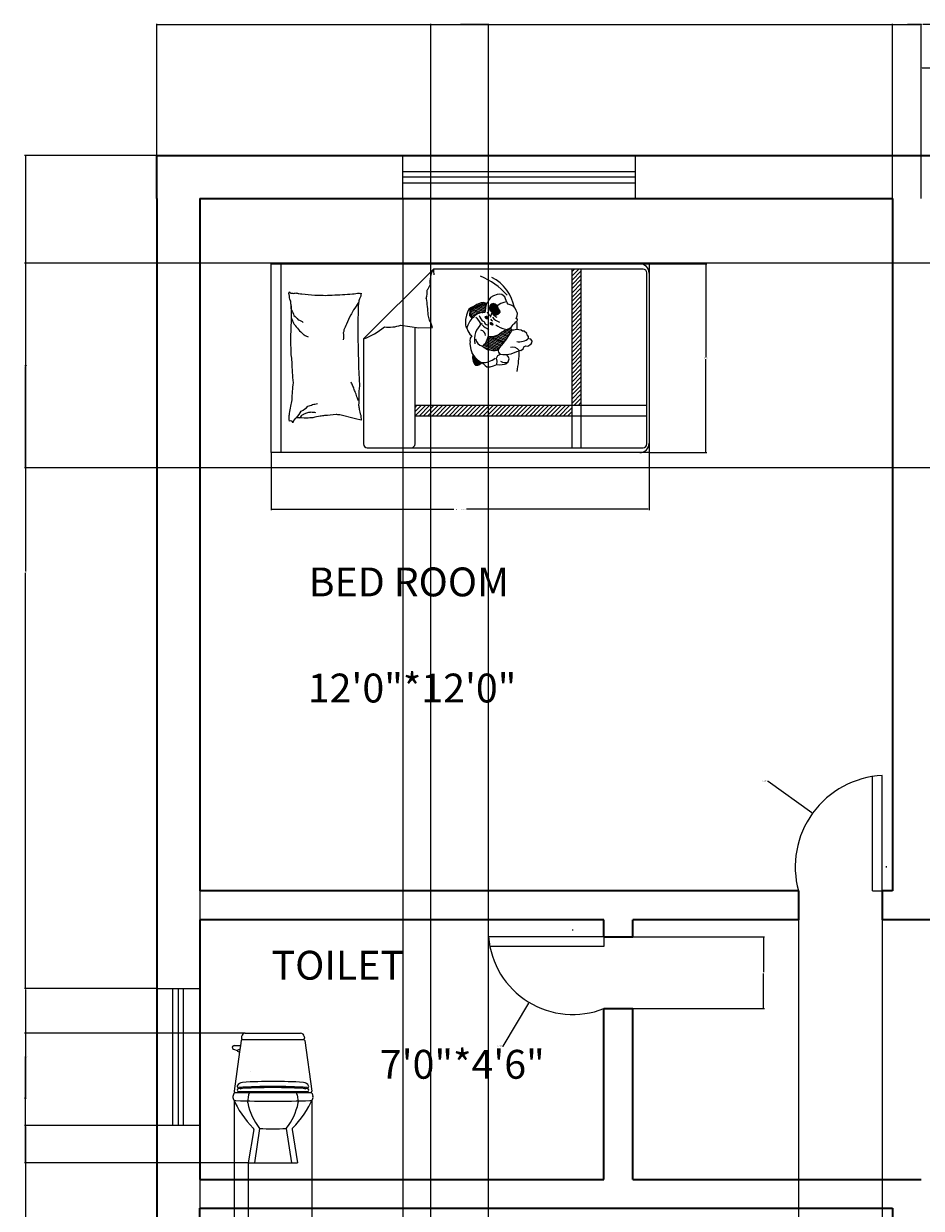
# Model space of a CAD drawing. Units: inches. Extents: x -17 to 1735, y -531 to 60.
# Tile 3 of 27: x -17 to 170, y -187 to 60. Entities that reach past the tile are written whole.
import ezdxf

# ---------------------------------------------------------------- set-up
doc = ezdxf.new("R2010")
doc.units = ezdxf.units.IN
doc.header["$MEASUREMENT"] = 0
for name, color, linetype, lineweight in [('A-ANNO-DIMS', 2, 'Continuous', 18), ('A-AREA-IDEN', 7, 'Continuous', 25), ('A-DOOR', 4, 'Continuous', 18), ('A-GLAZ', 4, 'Continuous', 18), ('A-WALL', 7, 'Continuous', 35)]:
    doc.layers.add(name, color=color, linetype=linetype, lineweight=lineweight)
for name, color, linetype, lineweight, true_color in [('A-FURN', 242, 'Continuous', 18, 0xcd2027), ('WC-Detail_dwgmodels.com', 30, 'Continuous', 13, 0xf8991e), ('WC-Outline_dwgmodels.com', 30, 'Continuous', 18, 0xf8991e)]:
    doc.layers.add(name, color=color, linetype=linetype, lineweight=lineweight, true_color=true_color)
doc.styles.get("Standard").update_dxf_attribs({"font": 'arial.ttf'})
doc.dimstyles.get("Standard").update_dxf_attribs({"dimtxt": 0.18, "dimasz": 0.18, "dimexe": 0.18, "dimexo": 0.0625, "dimgap": 0.09, "dimtad": 0, "dimtih": 1, "dimtoh": 1, "dimdec": 4, "dimzin": 0, "dimdsep": 46, "dimtxsty": 'Standard', "dimcen": 0.09, "dimadec": 0, "dimazin": 0, "dimtfac": 1, "dimtdec": 4, "dimtofl": 0, "dimtmove": 0, "dimatfit": 3, "dimfxl": 1, "dimtolj": 1, "dimtzin": 0, "dimarcsym": 0})

# ---------------------------------------------------------------- blocks, each defined once
blk = doc.blocks.new('BED-SINGLE-PLAN')
h = blk.add_hatch()
h.set_pattern_fill('ANSI31', color=256, scale=0.196463, angle=90, style=0)
h.set_pattern_definition([(225, (-27.0618, 48.5235), (-0.4410725, 0.4410725), [])])
h.paths.add_polyline_path([(62.55, 9.8), (29.91, 9.8), (29.91, 7.6), (62.55, 7.6)])
h.paths.add_polyline_path([(62.55, 9.8), (64.48, 9.8), (64.48, 38.18), (62.55, 38.18)])
h = blk.add_hatch()
h.set_pattern_fill('ANSI31', color=256, scale=2.357559, angle=112.8083, style=0)
h.set_pattern_definition([(157.808265, (-756.06988, 363.93155), (-0.11130837, -0.27286535), [])])
h.paths.add_polyline_path([(42.9, 28.85), (43.53, 29.05), (44.41, 29.13), (44.47, 29.42), (44.54, 30.16), (44.69, 30.7), (44.07, 30.85), (43.35, 30.52), (41.94, 30.01), (41.58, 29.54), (41.52, 28.62), (41.97, 28.11), (42.32, 28.49)])
h.paths.add_polyline_path([(45.09, 24.15, -0.19505), (43.9, 22.11, 0.242355), (47, 21.35, 0.070869), (50.1, 25.47), (49.89, 25.73), (49.62, 25.88), (48.82, 25.54), (47.87, 25.05), (47.21, 24.51), (46.36, 24.21)])
h = blk.add_hatch()
h.set_pattern_fill('ANSI31', color=256, scale=1.392433, angle=112.8083, style=0)
h.set_pattern_definition([(157.808265, (-714.60694, 367.20017), (-0.065741506, -0.161161097), [])])
h.paths.add_polyline_path([(45.75, 29.39), (46.01, 28.9), (46.14, 28.75), (46.34, 28.64), (46.5, 28.59), (46.86, 28.63), (47.26, 28.84), (47.59, 29.2), (47.52, 29.53), (47.21, 29.96), (47.12, 30.29), (46.97, 30.53), (46.54, 30.87), (46.19, 31), (45.76, 30.88), (45.45, 30.56), (45.37, 30.21), (45.4, 29.92), (45.54, 29.52)])
h = blk.add_hatch()
h.set_pattern_fill('ANSI31', color=256, scale=0.556973, angle=112.8083, style=0)
h.set_pattern_definition([(157.808265, (-714.60694, 367.20017), (-0.0262966024, -0.0644644387), [])])
h.paths.add_polyline_path([(45.8, 27.02), (45.59, 27), (45.47, 26.92), (45.58, 26.73), (45.73, 26.62), (46.03, 26.56), (46.14, 26.64), (46.08, 26.8), (45.97, 26.95)])
h.paths.add_polyline_path([(44.84, 28.32), (44.68, 28.33), (44.51, 28.27), (44.45, 28.18), (44.46, 28.11), (44.56, 28.01), (44.67, 27.9), (44.88, 27.87), (45.01, 27.95), (45.02, 28.12)])
h = blk.add_hatch()
h.set_pattern_fill('ANSI31', color=256, scale=1.178779, angle=112.8083, style=0)
h.set_pattern_definition([(157.808265, (-756.06988, 363.93155), (-0.055654185, -0.136432674), [])])
h.paths.add_polyline_path([(41.9, 20.41), (41.91, 20.39), (41.88, 19.75), (42, 19.04), (42.19, 18.52), (42.51, 18.19), (42.99, 18.18), (43.33, 18.35), (43.64, 18.6), (43.79, 18.72, -0.129501)])
for p, q in [((0, 39.29), (78.59, 39.29)), ((0, 0), (0, 39.29)), ((2.06, 0), (2.06, 39.29)), ((19.2, 23.68), (33.73, 38.18)), ((77.32, 38.18), (33.73, 38.18)), ((62.55, 1.01), (62.55, 38.18)), ((64.48, 1.01), (64.48, 38.18)), ((78.11, 1.8), (78.11, 37.39)), ((78.59, 39.29), (78.59, 0)), ((29.91, 1.8), (29.91, 26.11)), ((19.2, 23.68), (19.2, 1.8)), ((78.59, 0), (0, 0)), ((19.98, 1.01), (77.32, 1.01))]:
    blk.add_line(p, q)
for points in [[(5.25, 7.27, 0.263368), (4.51, 6.17, 0.494818), (3.78, 6.53, 0.049225), (3.71, 7.23, 0.036831), (3.78, 8.16, 0.031893), (4.1, 9.65, -0.035782), (4.37, 10.98, -0.032941), (4.6, 14.51, -0.026564), (4.37, 18.88, -0.017905), (4.16, 20.35, 0.009667), (4.07, 23.11, 0.03204), (4.1, 24.57, -0.018442), (4.22, 27.09, -0.010837), (4.19, 29.64, -0.014624), (4.07, 31.52, -0.111249), (3.78, 32.41, 0.153708), (3.63, 33.07, 0.076444), (3.7, 33.36, 0.215512), (3.78, 33.44, 0.585858), (3.9, 33.33, -0.363489), (4, 33.14, -0.191716), (4.45, 33.14, 0.129675), (5.1, 33.22, 0.01735), (5.76, 33.1, -0.019326), (6.36, 33, -0.018818), (9.04, 32.74, -0.021828), (11.37, 32.7, -0.006204), (12.7, 32.76, -0.001963), (16.9, 33, -0.028341), (18.32, 33.16, 0.117014), (18.67, 33.14, 0.36606), (18.71, 33.09, 0.03973), (18.6, 32.55, 0.048309), (18.38, 32.01, -0.062981), (18.23, 31.59, -0.04058), (18.09, 30.67, -0.014345), (18.01, 28.05, -0.005484), (18.04, 23.12, -0.004707), (18.15, 17.38, -0.008762), (18.26, 15.71, 0.008153), (18.38, 13.91, 0.06251), (18.2, 11.67, -0.078669), (18.12, 9.88, -0.047825), (18.31, 9, 0.034494), (18.6, 7.79, 0.023571), (18.71, 6.79, 0.510228), (18.67, 6.76), (17.49, 7.05), (14.25, 7.86, -0.073041), (13.48, 7.94, -0.023305), (11.08, 7.72, -0.018299), (10.18, 7.56, 0.01097), (8.68, 7.27, 0.042281), (7.34, 7.15, 0.027201), (5.24, 7.27)], [(4, 31.08, -0.088153), (4.14, 29.72, -0.088153), (4.73, 28.5, -0.077547), (5.58, 27.64, -0.077547), (6.65, 27.09)], [(18.15, 31.23, -0.016108), (17.12, 29.7, -0.024599), (16.53, 28.64, -0.009477), (15.62, 26.72, -0.015937), (15.13, 25.54, -0.072521), (14.99, 24.9, -0.033339), (14.98, 23.48)], [(4.22, 27.86, -0.027842), (4.64, 26.92, -0.048685), (4.96, 26.43, -0.023666), (5.91, 25.33, -0.031223), (6.72, 24.58, -0.046801), (7.03, 24.38, -0.023191), (7.68, 24.07)], [(19.2, 23.68, 0.085272), (23.52, 26.17, 0.124044), (26.96, 26.53), (30.71, 25.99), (33.56, 26.06)], [(18.09, 10.82, -0.009729), (17.74, 11.9, -0.009729), (17.34, 12.95, -0.007971), (16.99, 13.81, -0.007971), (16.61, 14.65)], [(5.25, 7.27, 0.077379), (6.25, 8.63, 0.077379), (7.61, 9.63, 0.047525), (8.58, 10.02, 0.047525), (9.6, 10.22)], [(5.88, 7.21, 0.05369), (6.39, 7.77, 0.070312), (6.87, 8.08, 0.015448), (7.21, 8.23, 0.013244), (7.61, 8.38, 0.082127), (8.32, 8.5, 0.064164), (9.23, 8.38)]]:
    blk.add_lwpolyline(points, format="xyb")
for points in [[(43.79, 18.72), (44.04, 18.56), (44.46, 18.12), (44.86, 17.87), (45.53, 17.83), (46.24, 18.04), (46.92, 18.32), (47.57, 18.24), (48.51, 18.4), (48.81, 18.47), (49.3, 18.91), (49.47, 19.49), (49.29, 19.97), (48.92, 20.38), (49.91, 20.56), (51.05, 21.01), (51.55, 21.16), (51.59, 21.33), (51.88, 21.27), (52.46, 21.66), (52.55, 22), (52.94, 22.19), (53.35, 22.15), (53.8, 22.4), (54.07, 22.6), (54.21, 22.84), (54.27, 23.19), (53.95, 23.59), (53.59, 23.67), (53.53, 23.82), (53.51, 24.14), (53.22, 24.49), (53.14, 24.75), (52.57, 25.26), (52.25, 25.24), (51.94, 25.49), (50.98, 25.59), (50.47, 25.47), (50.13, 25.44), (49.89, 25.73), (49.62, 25.88), (49.97, 26.17), (50.19, 26.42), (50.21, 26.66), (50.65, 26.93), (50.88, 27.18), (51.12, 27.37), (51.24, 27.65), (51.14, 27.82), (50.96, 27.83), (50.98, 28.05), (51.12, 28.43), (51.19, 28.96), (51.17, 29.16), (50.93, 29.59), (50.71, 30.03), (50.42, 30.38), (49.9, 30.7), (49.25, 30.9), (49.09, 31.16), (48.83, 31.61), (48.74, 31.98), (48.58, 32.42), (47.95, 32.87), (47.57, 32.94), (46.99, 32.91), (46.24, 32.59), (45.6, 32.26), (45.31, 31.84), (44.99, 31.21), (44.78, 31), (44.17, 31.25), (43.66, 31.18), (42.75, 30.83), (42.33, 30.56), (41.65, 30.22), (41.1, 29.84), (40.84, 29.19), (40.62, 28.57), (40.38, 27.67), (40.38, 26.55), (40.44, 26.19), (40.7, 25.86), (40.89, 25.34), (41.33, 24.64), (41.74, 24.31), (41.36, 23.8), (41.32, 23.27), (41.4, 23.13), (41.29, 22.64), (41.54, 21.48), (41.64, 21.02), (41.71, 20.72), (41.85, 20.54), (41.91, 20.39), (41.88, 19.75), (42, 19.04), (42.19, 18.52), (42.51, 18.19), (42.99, 18.18), (43.33, 18.35), (43.64, 18.6), (43.79, 18.72)], [(41.81, 27.96), (41.3, 28.55), (41.37, 29.62), (41.81, 30.2), (43.27, 30.72), (44.05, 31.08), (44.74, 30.91)], [(41.97, 28.11), (41.52, 28.62), (41.58, 29.54), (41.94, 30.01), (43.35, 30.52), (44.07, 30.85), (44.69, 30.7)], [(44.78, 31), (44.54, 30.16), (44.47, 29.42), (44.41, 29.13), (43.53, 29.05), (42.9, 28.85), (42.32, 28.49), (41.97, 28.11)], [(45.75, 29.39), (46.01, 28.9), (46.14, 28.75), (46.34, 28.64), (46.5, 28.59), (46.86, 28.63), (47.26, 28.84), (47.59, 29.2), (47.52, 29.53), (47.21, 29.96), (47.12, 30.29), (46.97, 30.53), (46.54, 30.87), (46.19, 31), (45.76, 30.88), (45.45, 30.56), (45.37, 30.21), (45.4, 29.92), (45.54, 29.52), (45.75, 29.39)], [(44.67, 27.9), (44.88, 27.87), (45.01, 27.95), (45.02, 28.12), (44.84, 28.32), (44.68, 28.33), (44.51, 28.27), (44.45, 28.18), (44.46, 28.11), (44.56, 28.01), (44.67, 27.9)], [(45.09, 24.15), (46.36, 24.21), (47.21, 24.51), (47.87, 25.05), (48.82, 25.54), (49.62, 25.88)], [(45.73, 26.62), (46.03, 26.56), (46.14, 26.64), (46.08, 26.8), (45.97, 26.95), (45.8, 27.02), (45.59, 27), (45.47, 26.92), (45.58, 26.73), (45.73, 26.62)], [(46.92, 18.32), (46.96, 18.99), (46.83, 19.65), (47.14, 20.19), (47.67, 20.47), (48.14, 20.41), (48.92, 20.38)], [(78.11, 9.8), (29.91, 9.8)], [(78.11, 7.6), (29.91, 7.6)]]:
    blk.add_lwpolyline(points)
for centre, radius, start, end in [((38, 35.55), 5.01, 148.4201, 187.4443), ((39.59, 38.03), 5.86, 178.5957, 190.5745), ((76.62, 37.33), 1.96, 0, 90), ((77.32, 37.39), 0.786, 0, 90), ((30.16, 35.71), 2.97, 320.6139, 344.2839), ((38.03, 23.16), 14.6, 41.0314, 67.8934), ((42.02, 28.67), 8.66, 9.4371, 63.5432), ((26.72, 33.64), 5.74, 344.2839, 1.7887), ((10.08, 27.94), 22.56, 1.7887, 10.5945), ((49.55, 27.35), 4.08, 98.3054, 168.9473), ((46.45, 29.64), 0.695, 97.7782, 185.1837), ((45.99, 30.23), 0.379, 14.3938, 104.927), ((46.73, 29.37), 0.572, 4.9536, 167.0589), ((46.6, 29.87), 0.512, 10.7395, 118.1073), ((26.25, 26.33), 6.78, 10.5945, 19.9478), ((19.4, 20.92), 15.06, 19.9478, 26.2172), ((44.35, 25.28), 3.69, 130.0646, 171.0184), ((40.73, 25.75), 3, 17.6284, 51.9822), ((45.01, 28.9), 1.81, 191.014, 241.9838), ((44.99, 27.32), 0.729, 184.2478, 266.558), ((46.38, 29.75), 1.54, 196.6236, 237.032), ((46.1, 27.86), 0.431, 180.1097, 257.3601), ((48.22, 29.75), 2.7, 214.8006, 254.2713), ((54.94, 39.79), 14.12, 231.9927, 235.4886), ((11.77, 25.26), 39.39, 0.4734, 3.0628), ((46.27, 23.6), 4.03, 126.6141, 193.9334), ((43.31, 24.26), 1.25, 5.5542, 75.9589), ((47.07, 29.65), 4.44, 223.4778, 246.0857), ((49.36, 29.79), 4.14, 230.1138, 260.2426), ((34.07, 34.29), 18.29, 314.9707, 331.1855), ((44.61, 24.23), 2.23, 194.7325, 251.4551), ((41.98, 24.59), 3.13, 307.7547, 351.9024), ((51.66, 25.7), 2.65, 256.5554, 314.9062), ((46.04, 23.16), 4.97, 209.3586, 243.0552), ((46.2, 24.74), 3.49, 228.8697, 283.3627), ((48.1, 21.24), 0.883, 163.0797, 240.2757), ((50.18, 20.2), 1.73, 36.8303, 104.4951), ((29.44, 21.14), 22.11, 348.8153, 0.0463), ((44.02, 22.54), 3.83, 266.6283, 311.5254), ((48.58, 20.29), 1.56, 234.8325, 297.5513), ((19.98, 1.8), 0.786, 180, 270), ((29.12, 1.8), 0.786, 270, 0), ((76.62, 1.96), 1.96, 270, 0), ((77.32, 1.8), 0.786, 270, 0)]:
    blk.add_arc(centre, radius, start, end)
blk = doc.blocks.new('WIN-FRAME-48IN')
for p, q in [((3.31, 48.33), (3.31, 0)), ((5.59, 0), (5.59, 48.33))]:
    blk.add_line(p, q)
blk.add_lwpolyline([(0, 48.33), (9, 48.33), (9, 0), (0, 0)], close=True)
blk = doc.blocks.new('*D7')
at = {"layer": 'A-ANNO-DIMS', "color": 0, "lineweight": -2, "transparency": 16777216}
for p, q in [((34.88, -29.66), (34.88, -41.56)), ((113.46, -29.66), (113.46, -41.56)), ((35.06, -41.38), (72.85, -41.38)), ((113.28, -41.38), (75.49, -41.38))]:
    blk.add_line(p, q, dxfattribs=at)
at = {"layer": 'A-ANNO-DIMS', "color": 0, "transparency": 16777216}
for points in [[(35.06, -41.35), (35.06, -41.41), (34.88, -41.38)], [(113.28, -41.35), (113.28, -41.41), (113.46, -41.38)]]:
    blk.add_solid(points, dxfattribs=at)
at = {"layer": 'Defpoints', "color": 0, "transparency": 16777216}
for p in [(34.88, -29.59), (113.46, -29.59), (113.46, -41.38)]:
    blk.add_point(p, dxfattribs=at)
at = {"layer": 'A-ANNO-DIMS', "color": 0, "transparency": 16777216, "insert": (74.17, -41.38), "char_height": 0.18, "attachment_point": 5}
blk.add_mtext('\\A1;SINGLE BED 79 TYP.', dxfattribs=at)
blk = doc.blocks.new('*D8')
at = {"layer": 'A-ANNO-DIMS', "color": 0, "lineweight": -2, "transparency": 16777216}
for p, q in [((113.53, 9.7), (125.43, 9.7)), ((125.25, 9.52), (125.25, -9.76)), ((125.25, -29.41), (125.25, -10.13)), ((113.53, -29.59), (125.43, -29.59))]:
    blk.add_line(p, q, dxfattribs=at)
at = {"layer": 'A-ANNO-DIMS', "color": 0, "transparency": 16777216}
for points in [[(125.22, 9.52), (125.28, 9.52), (125.25, 9.7)], [(125.22, -29.41), (125.28, -29.41), (125.25, -29.59)]]:
    blk.add_solid(points, dxfattribs=at)
at = {"layer": 'Defpoints', "color": 0, "transparency": 16777216}
for p in [(113.46, 9.7), (125.25, 9.7), (113.46, -29.59)]:
    blk.add_point(p, dxfattribs=at)
at = {"layer": 'A-ANNO-DIMS', "color": 0, "transparency": 16777216, "insert": (125.25, -9.95), "char_height": 0.18, "attachment_point": 5}
blk.add_mtext('\\A1;39 TYP.', dxfattribs=at)
blk = doc.blocks.new('*D9')
at = {"layer": 'A-ANNO-DIMS', "color": 0, "lineweight": -2, "transparency": 16777216}
for p, q in [((11.06, 32.29), (11.06, 59.62)), ((11.24, 59.44), (169.77, 59.44)), ((328.88, 59.44), (170.35, 59.44)), ((329.06, 32.29), (329.06, 59.62))]:
    blk.add_line(p, q, dxfattribs=at)
at = {"layer": 'A-ANNO-DIMS', "color": 0, "transparency": 16777216}
for points in [[(11.24, 59.47), (11.24, 59.41), (11.06, 59.44)], [(328.88, 59.47), (328.88, 59.41), (329.06, 59.44)]]:
    blk.add_solid(points, dxfattribs=at)
at = {"layer": 'Defpoints', "color": 0, "transparency": 16777216}
for p in [(329.06, 59.44), (11.06, 32.23), (329.06, 32.23)]:
    blk.add_point(p, dxfattribs=at)
at = {"layer": 'A-ANNO-DIMS', "color": 0, "transparency": 16777216, "insert": (170.06, 59.44), "char_height": 0.18, "attachment_point": 5}
blk.add_mtext('\\A1;318', dxfattribs=at)
blk = doc.blocks.new('*D11')
at = {"layer": 'A-ANNO-DIMS', "color": 0, "lineweight": -2, "transparency": 16777216}
for p, q in [((20.06, 23.17), (20.06, -531.46)), ((62.23, 23.17), (62.23, -531.46)), ((20.24, -531.28), (40.75, -531.28)), ((62.05, -531.28), (41.54, -531.28))]:
    blk.add_line(p, q, dxfattribs=at)
at = {"layer": 'A-ANNO-DIMS', "color": 0, "transparency": 16777216}
for points in [[(20.24, -531.25), (20.24, -531.31), (20.06, -531.28)], [(62.05, -531.25), (62.05, -531.31), (62.23, -531.28)]]:
    blk.add_solid(points, dxfattribs=at)
at = {"layer": 'Defpoints', "color": 0, "transparency": 16777216}
for p in [(20.06, 23.23), (62.23, 23.23), (62.23, -531.28)]:
    blk.add_point(p, dxfattribs=at)
at = {"layer": 'A-ANNO-DIMS', "color": 0, "transparency": 16777216, "insert": (41.15, -531.28), "char_height": 0.18, "attachment_point": 5}
blk.add_mtext('\\A1;42.17', dxfattribs=at)
blk = doc.blocks.new('*D13')
at = {"layer": 'A-ANNO-DIMS', "color": 0, "lineweight": -2, "transparency": 16777216}
for p, q in [((11, 32.23), (-16.4, 32.23)), ((-16.22, 32.05), (-16.22, -54.24)), ((-16.22, -140.9), (-16.22, -54.61)), ((11, -141.08), (-16.4, -141.08))]:
    blk.add_line(p, q, dxfattribs=at)
at = {"layer": 'A-ANNO-DIMS', "color": 0, "transparency": 16777216}
for points in [[(-16.25, 32.05), (-16.19, 32.05), (-16.22, 32.23)], [(-16.25, -140.9), (-16.19, -140.9), (-16.22, -141.08)]]:
    blk.add_solid(points, dxfattribs=at)
at = {"layer": 'Defpoints', "color": 0, "transparency": 16777216}
for p in [(11.06, 32.23), (-16.22, -141.08), (11.06, -141.08)]:
    blk.add_point(p, dxfattribs=at)
at = {"layer": 'A-ANNO-DIMS', "color": 0, "transparency": 16777216, "insert": (-16.22, -54.42), "char_height": 0.18, "attachment_point": 5}
blk.add_mtext('\\A1;173.3', dxfattribs=at)
blk = doc.blocks.new('*D14')
at = {"layer": 'A-ANNO-DIMS', "color": 0, "lineweight": -2, "transparency": 16777216}
for p, q in [((11, -141.08), (-16.4, -141.08)), ((-16.22, -141.26), (-16.22, -155.13)), ((-16.22, -169.37), (-16.22, -155.49)), ((11, -169.55), (-16.4, -169.55))]:
    blk.add_line(p, q, dxfattribs=at)
at = {"layer": 'A-ANNO-DIMS', "color": 0, "transparency": 16777216}
for points in [[(-16.25, -141.26), (-16.19, -141.26), (-16.22, -141.08)], [(-16.25, -169.37), (-16.19, -169.37), (-16.22, -169.55)]]:
    blk.add_solid(points, dxfattribs=at)
at = {"layer": 'Defpoints', "color": 0, "transparency": 16777216}
for p in [(11.06, -141.08), (-16.22, -169.55), (11.06, -169.55)]:
    blk.add_point(p, dxfattribs=at)
at = {"layer": 'A-ANNO-DIMS', "color": 0, "transparency": 16777216, "insert": (-16.22, -155.31), "char_height": 0.18, "attachment_point": 5}
blk.add_mtext('\\A1;28.467', dxfattribs=at)
blk = doc.blocks.new('*D15')
at = {"layer": 'A-ANNO-DIMS', "color": 0, "lineweight": -2, "transparency": 16777216}
for p, q in [((11, -169.55), (-16.4, -169.55)), ((-16.22, -169.73), (-16.22, -196.03)), ((-16.22, -222.7), (-16.22, -196.39)), ((11, -222.88), (-16.4, -222.88))]:
    blk.add_line(p, q, dxfattribs=at)
at = {"layer": 'A-ANNO-DIMS', "color": 0, "transparency": 16777216}
for points in [[(-16.25, -169.73), (-16.19, -169.73), (-16.22, -169.55)], [(-16.25, -222.7), (-16.19, -222.7), (-16.22, -222.88)]]:
    blk.add_solid(points, dxfattribs=at)
at = {"layer": 'Defpoints', "color": 0, "transparency": 16777216}
for p in [(11.06, -169.55), (-16.22, -222.88), (11.06, -222.88)]:
    blk.add_point(p, dxfattribs=at)
at = {"layer": 'A-ANNO-DIMS', "color": 0, "transparency": 16777216, "insert": (-16.22, -196.21), "char_height": 0.18, "attachment_point": 5}
blk.add_mtext('\\A1;53.33', dxfattribs=at)
blk = doc.blocks.new('*D29')
at = {"layer": 'A-ANNO-DIMS', "color": 0, "lineweight": -2, "transparency": 16777216}
for p, q in [((164.06, 23.29), (164.06, 59.62)), ((164.24, 59.44), (166.91, 59.44)), ((169.88, 59.44), (167.21, 59.44)), ((170.06, 23.29), (170.06, 59.62))]:
    blk.add_line(p, q, dxfattribs=at)
at = {"layer": 'A-ANNO-DIMS', "color": 0, "transparency": 16777216}
for points in [[(164.24, 59.47), (164.24, 59.41), (164.06, 59.44)], [(169.88, 59.47), (169.88, 59.41), (170.06, 59.44)]]:
    blk.add_solid(points, dxfattribs=at)
at = {"layer": 'Defpoints', "color": 0, "transparency": 16777216}
for p in [(170.06, 59.44), (164.06, 23.23), (170.06, 23.23)]:
    blk.add_point(p, dxfattribs=at)
at = {"layer": 'A-ANNO-DIMS', "color": 0, "transparency": 16777216, "insert": (167.06, 59.44), "char_height": 0.18, "attachment_point": 5}
blk.add_mtext('\\A1;6', dxfattribs=at)
blk = doc.blocks.new('*D30')
at = {"layer": 'A-ANNO-DIMS', "color": 0, "lineweight": -2, "transparency": 16777216}
for p, q in [((144.53, -126.83), (144.53, -531.46)), ((161.94, -126.83), (161.94, -531.46)), ((144.71, -531.28), (152.87, -531.28)), ((161.76, -531.28), (153.6, -531.28))]:
    blk.add_line(p, q, dxfattribs=at)
at = {"layer": 'A-ANNO-DIMS', "color": 0, "transparency": 16777216}
for points in [[(144.71, -531.25), (144.71, -531.31), (144.53, -531.28)], [(161.76, -531.25), (161.76, -531.31), (161.94, -531.28)]]:
    blk.add_solid(points, dxfattribs=at)
at = {"layer": 'Defpoints', "color": 0, "transparency": 16777216}
for p in [(144.53, -126.77), (161.94, -126.77), (161.94, -531.28)]:
    blk.add_point(p, dxfattribs=at)
at = {"layer": 'A-ANNO-DIMS', "color": 0, "transparency": 16777216, "insert": (153.23, -531.28), "char_height": 0.18, "attachment_point": 5}
blk.add_mtext('\\A1;17.41', dxfattribs=at)
blk = doc.blocks.new('*D32')
at = {"layer": 'A-ANNO-DIMS', "color": 0, "lineweight": -2, "transparency": 16777216}
for p, q in [((110.12, -130.32), (137.44, -130.32)), ((137.26, -130.5), (137.26, -137.59)), ((137.26, -145.04), (137.26, -137.95)), ((110.12, -145.22), (137.44, -145.22))]:
    blk.add_line(p, q, dxfattribs=at)
at = {"layer": 'A-ANNO-DIMS', "color": 0, "transparency": 16777216}
for points in [[(137.23, -130.5), (137.29, -130.5), (137.26, -130.32)], [(137.23, -145.04), (137.29, -145.04), (137.26, -145.22)]]:
    blk.add_solid(points, dxfattribs=at)
at = {"layer": 'Defpoints', "color": 0, "transparency": 16777216}
for p in [(110.06, -130.32), (110.06, -145.22), (137.26, -145.22)]:
    blk.add_point(p, dxfattribs=at)
at = {"layer": 'A-ANNO-DIMS', "color": 0, "transparency": 16777216, "insert": (137.26, -137.77), "char_height": 0.18, "attachment_point": 5}
blk.add_mtext('\\A1;14.9', dxfattribs=at)
blk = doc.blocks.new('*D38')
at = {"layer": 'A-ANNO-DIMS', "color": 0, "lineweight": -2, "transparency": 16777216}
for p, q in [((222.23, 9.8), (-16.4, 9.8)), ((-16.22, 9.62), (-16.22, -11.31)), ((-16.22, -32.6), (-16.22, -11.67)), ((222.18, -32.78), (-16.4, -32.78))]:
    blk.add_line(p, q, dxfattribs=at)
at = {"layer": 'A-ANNO-DIMS', "color": 0, "transparency": 16777216}
for points in [[(-16.25, 9.62), (-16.19, 9.62), (-16.22, 9.8)], [(-16.25, -32.6), (-16.19, -32.6), (-16.22, -32.78)]]:
    blk.add_solid(points, dxfattribs=at)
at = {"layer": 'Defpoints', "color": 0, "transparency": 16777216}
for p in [(222.29, 9.8), (-16.22, -32.78), (222.24, -32.78)]:
    blk.add_point(p, dxfattribs=at)
at = {"layer": 'A-ANNO-DIMS', "color": 0, "transparency": 16777216, "insert": (-16.22, -11.49), "char_height": 0.18, "attachment_point": 5}
blk.add_mtext('\\A1;42.58', dxfattribs=at)
blk = doc.blocks.new('*D43')
at = {"layer": 'A-ANNO-DIMS', "color": 0, "lineweight": -2, "transparency": 16777216}
for p, q in [((170.06, 23.29), (170.06, 50.61)), ((170.24, 50.43), (244.78, 50.43)), ((319.88, 50.43), (245.34, 50.43)), ((320.06, 23.29), (320.06, 50.61))]:
    blk.add_line(p, q, dxfattribs=at)
at = {"layer": 'A-ANNO-DIMS', "color": 0, "transparency": 16777216}
for points in [[(170.24, 50.46), (170.24, 50.4), (170.06, 50.43)], [(319.88, 50.46), (319.88, 50.4), (320.06, 50.43)]]:
    blk.add_solid(points, dxfattribs=at)
at = {"layer": 'Defpoints', "color": 0, "transparency": 16777216}
for p in [(320.06, 50.43), (170.06, 23.23), (320.06, 23.23)]:
    blk.add_point(p, dxfattribs=at)
at = {"layer": 'A-ANNO-DIMS', "color": 0, "transparency": 16777216, "insert": (245.06, 50.43), "char_height": 0.18, "attachment_point": 5}
blk.add_mtext('\\A1;150', dxfattribs=at)
blk = doc.blocks.new('*D44')
at = {"layer": 'A-ANNO-DIMS', "color": 0, "lineweight": -2, "transparency": 16777216}
for p, q in [((29.42, -150.37), (-16.4, -150.37)), ((-16.22, -150.55), (-16.22, -163.67)), ((-16.22, -177.15), (-16.22, -164.03)), ((30.03, -177.33), (-16.4, -177.33))]:
    blk.add_line(p, q, dxfattribs=at)
at = {"layer": 'A-ANNO-DIMS', "color": 0, "transparency": 16777216}
for points in [[(-16.25, -150.55), (-16.19, -150.55), (-16.22, -150.37)], [(-16.25, -177.15), (-16.19, -177.15), (-16.22, -177.33)]]:
    blk.add_solid(points, dxfattribs=at)
at = {"layer": 'Defpoints', "color": 0, "transparency": 16777216}
for p in [(-16.22, -150.37), (29.48, -150.37), (30.1, -177.33)]:
    blk.add_point(p, dxfattribs=at)
at = {"layer": 'A-ANNO-DIMS', "color": 0, "transparency": 16777216, "insert": (-16.22, -163.85), "char_height": 0.18, "attachment_point": 5}
blk.add_mtext('\\A1;26.96', dxfattribs=at)
blk = doc.blocks.new('*D45')
at = {"layer": 'A-ANNO-DIMS', "color": 0, "lineweight": -2, "transparency": 16777216}
for p, q in [((27.16, -164.32), (27.16, -531.46)), ((43.3, -164.32), (43.3, -531.46)), ((27.34, -531.28), (34.85, -531.28)), ((43.12, -531.28), (35.62, -531.28))]:
    blk.add_line(p, q, dxfattribs=at)
at = {"layer": 'A-ANNO-DIMS', "color": 0, "transparency": 16777216}
for points in [[(27.34, -531.25), (27.34, -531.31), (27.16, -531.28)], [(43.12, -531.25), (43.12, -531.31), (43.3, -531.28)]]:
    blk.add_solid(points, dxfattribs=at)
at = {"layer": 'Defpoints', "color": 0, "transparency": 16777216}
for p in [(27.16, -164.25), (43.3, -164.25), (43.3, -531.28)]:
    blk.add_point(p, dxfattribs=at)
at = {"layer": 'A-ANNO-DIMS', "color": 0, "transparency": 16777216, "insert": (35.23, -531.28), "char_height": 0.18, "attachment_point": 5}
blk.add_mtext('\\A1;16.14', dxfattribs=at)
blk = doc.blocks.new('*D46')
at = {"layer": 'A-ANNO-DIMS', "color": 0, "lineweight": -2, "transparency": 16777216}
for p, q in [((30.1, -177.39), (30.1, -531.46)), ((20.06, -180.83), (20.06, -531.46)), ((20.24, -531.28), (24.62, -531.28)), ((29.92, -531.28), (25.53, -531.28))]:
    blk.add_line(p, q, dxfattribs=at)
at = {"layer": 'A-ANNO-DIMS', "color": 0, "transparency": 16777216}
for points in [[(20.24, -531.25), (20.24, -531.31), (20.06, -531.28)], [(29.92, -531.25), (29.92, -531.31), (30.1, -531.28)]]:
    blk.add_solid(points, dxfattribs=at)
at = {"layer": 'Defpoints', "color": 0, "transparency": 16777216}
for p in [(30.1, -177.33), (20.06, -180.77), (30.1, -531.28)]:
    blk.add_point(p, dxfattribs=at)
at = {"layer": 'A-ANNO-DIMS', "color": 0, "transparency": 16777216, "insert": (25.08, -531.28), "char_height": 0.18, "attachment_point": 5}
blk.add_mtext('\\A1;10.034', dxfattribs=at)
blk = doc.blocks.new('*D50')
at = {"layer": 'A-ANNO-DIMS', "color": 0, "lineweight": -2, "transparency": 16777216}
for p, q in [((68.06, -417.02), (68.06, 59.62)), ((68.24, 59.44), (73.85, 59.44)), ((79.88, 59.44), (74.27, 59.44)), ((80.06, -417.02), (80.06, 59.62))]:
    blk.add_line(p, q, dxfattribs=at)
at = {"layer": 'A-ANNO-DIMS', "color": 0, "transparency": 16777216}
for points in [[(68.24, 59.47), (68.24, 59.41), (68.06, 59.44)], [(79.88, 59.47), (79.88, 59.41), (80.06, 59.44)]]:
    blk.add_solid(points, dxfattribs=at)
at = {"layer": 'Defpoints', "color": 0, "transparency": 16777216}
for p in [(80.06, 59.44), (68.06, -417.08), (80.06, -417.08)]:
    blk.add_point(p, dxfattribs=at)
at = {"layer": 'A-ANNO-DIMS', "color": 0, "transparency": 16777216, "insert": (74.06, 59.44), "char_height": 0.18, "attachment_point": 5}
blk.add_mtext('\\A1;12', dxfattribs=at)
blk = doc.blocks.new('*D53')
at = {"layer": 'A-ANNO-DIMS', "color": 0, "lineweight": -2, "transparency": 16777216}
for p, q in [((138.07, -97.9), (138.25, -97.9)), ((138.25, -97.9), (147.31, -104.47)), ((162.72, -115.72), (162.9, -115.72)), ((162.81, -115.81), (162.81, -115.63))]:
    blk.add_line(p, q, dxfattribs=at)
at = {"layer": 'A-ANNO-DIMS', "color": 0, "transparency": 16777216}
blk.add_solid([(147.33, -104.45), (147.29, -104.5), (147.46, -104.58)], dxfattribs=at)
at = {"layer": 'Defpoints', "color": 0, "transparency": 16777216}
for p in [(147.46, -104.58), (162.81, -115.72)]:
    blk.add_point(p, dxfattribs=at)
at = {"layer": 'A-ANNO-DIMS', "color": 0, "transparency": 16777216, "insert": (137.52, -97.9), "char_height": 0.18, "attachment_point": 5}
blk.add_mtext('\\A1;R18.967', dxfattribs=at)
blk = doc.blocks.new('*D55')
at = {"layer": 'A-ANNO-DIMS', "color": 0, "lineweight": -2, "transparency": 16777216}
for p, q in [((97.49, -128.88), (97.67, -128.88)), ((97.58, -128.97), (97.58, -128.79)), ((83.14, -153.01), (88.46, -144.12)), ((82.96, -153.01), (83.14, -153.01))]:
    blk.add_line(p, q, dxfattribs=at)
at = {"layer": 'A-ANNO-DIMS', "color": 0, "transparency": 16777216}
blk.add_solid([(88.44, -144.1), (88.49, -144.13), (88.56, -143.96)], dxfattribs=at)
at = {"layer": 'Defpoints', "color": 0, "transparency": 16777216}
for p in [(97.58, -128.88), (88.56, -143.96)]:
    blk.add_point(p, dxfattribs=at)
at = {"layer": 'A-ANNO-DIMS', "color": 0, "transparency": 16777216, "insert": (82.41, -153.01), "char_height": 0.18, "attachment_point": 5}
blk.add_mtext('\\A1;R17.582', dxfattribs=at)

msp = doc.modelspace()

# ---------------------------------------------------------------- linework, layer by layer
at = {"layer": 'A-DOOR'}
for p, q in [((159.9382, -120.7685), (159.9382, -96.967)), ((161.9382, -120.7685), (161.9382, -96.7685)), ((159.9382, -120.7685), (161.9382, -120.7685)), ((104.0618, -130.3218), (80.0618, -130.3218)), ((104.0618, -130.3218), (104.0618, -132.3218)), ((104.0618, -132.3218), (80.3433, -132.3218))]:
    msp.add_line(p, q, dxfattribs=at)
for centre, radius, start, end in [((162.809, -115.7152), 18.9667, 92.631405, 195.451747), ((97.5841, -128.8755), 17.5819, 184.718615, 291.618619)]:
    msp.add_arc(centre, radius, start, end, dxfattribs=at)
at = {"layer": 'A-GLAZ'}
for p, q in [((62.2307, 27.7457), (110.5565, 27.7457)), ((14.3729, -141.0795), (14.3729, -169.5467)), ((15.5058, -141.0795), (15.5058, -169.5467)), ((16.6545, -169.5467), (16.6545, -141.0795)), ((20.0618, -169.5467), (11.0618, -169.5467))]:
    msp.add_line(p, q, dxfattribs=at)
msp.add_lwpolyline([(11.0618, -169.5467), (11.0618, -141.0795), (20.0618, -141.0795), (20.0618, -169.5467)], dxfattribs=at)
at = {"layer": 'A-WALL'}
for p, q in [((11.0618, 32.2315), (320.0618, 32.2315)), ((11.0618, 23.2315), (11.0618, 32.2315)), ((11.0618, 23.2315), (11.0618, -141.0795)), ((20.0618, 23.2315), (164.0618, 23.2315)), ((20.0618, 23.2315), (20.0618, -120.7685)), ((164.0618, 23.2315), (164.0618, -120.7685)), ((144.5278, -120.7685), (20.0618, -120.7685)), ((144.5278, -120.7685), (144.5278, -126.7685)), ((164.0618, -120.7685), (161.9382, -120.7685)), ((161.9382, -120.7685), (161.9382, -126.7685)), ((104.0618, -126.7685), (20.0618, -126.7685)), ((104.0618, -126.7685), (20.0618, -126.7685)), ((20.0618, -126.7685), (20.0618, -141.0795)), ((104.0618, -130.3218), (104.0618, -126.7685)), ((144.5278, -126.7685), (110.0618, -126.7685)), ((144.5278, -126.7685), (110.0618, -126.7685)), ((110.0618, -130.3218), (110.0618, -126.7685)), ((164.0618, -126.7685), (161.9382, -126.7685)), ((172.5508, -126.7685), (161.9382, -126.7685)), ((104.0618, -130.3218), (110.0618, -130.3218)), ((11.0618, -141.0795), (11.0618, -195.0795)), ((20.0618, -141.0795), (20.0618, -180.7685)), ((104.0618, -180.7685), (104.0618, -145.2207)), ((104.0618, -145.2207), (110.0618, -145.2207)), ((110.0618, -180.7685), (110.0618, -145.2207)), ((20.0618, -180.7685), (104.0618, -180.7685)), ((20.0618, -180.7685), (104.0618, -180.7685)), ((110.0618, -180.7685), (170.0618, -180.7685)), ((20.0618, -186.7685), (104.0618, -186.7685)), ((20.0618, -186.7685), (164.0618, -186.7685)), ((20.0618, -195.0795), (20.0618, -186.7685)), ((164.0618, -186.7685), (164.0618, -296.302))]:
    msp.add_line(p, q, dxfattribs=at)
at = {"layer": 'WC-Detail_dwgmodels.com'}
for p, q in [((28.9311, -151.6558), (41.5313, -151.6558)), ((30.659, -158.287), (30.659, -158.287)), ((28.0422, -162.4392), (42.4202, -162.4392)), ((28.3196, -162.4392), (28.3196, -162.5676)), ((29.5625, -162.4392), (29.5625, -162.5676)), ((40.8998, -162.4392), (40.8998, -162.5676)), ((42.1428, -162.4392), (42.1428, -162.5676)), ((30.1839, -163.1399), (29.973, -164.6803)), ((40.2785, -163.1399), (40.4893, -164.6803)), ((32.4524, -170.148), (31.4003, -177.3307)), ((38.01, -170.148), (39.0621, -177.3307))]:
    msp.add_line(p, q, dxfattribs=at)
for centre, radius, start, end in [((28.4549, -154.6918), 0.987, 95.774795, 132.710831), ((28.0422, -162.1825), 0.2567, 94.090817, 270), ((35.2312, -262.6996), 101.0306, 85.909183, 94.090817), ((28.5241, -161.6801), 0.2113, 171.42998, 16.167118), ((28.4479, -162.5676), 0.1284, 180, 270), ((29.4342, -162.5676), 0.1284, 270, 0), ((41.0282, -162.5676), 0.1284, 180, 270), ((41.9383, -161.6801), 0.2113, 163.832882, 8.57002), ((42.0144, -162.5676), 0.1284, 270, 0), ((42.4202, -162.1825), 0.2567, 270, 85.909183), ((27.5491, -163.7156), 0.6622, 200.13709, 268.27943), ((35.2312, 92.0242), 256.5175, 268.27943, 271.72057), ((30.4818, -164.75), 0.5135, 172.20623, 192.973077), ((42.6739, -162.1476), 12.9802, 192.085483, 218.050565), ((30.6926, -163.2095), 0.5135, 90, 172.20623), ((27.7885, -162.1476), 12.9802, 321.949435, 347.914517), ((39.7697, -163.2095), 0.5135, 7.79377, 90), ((39.9806, -164.75), 0.5135, 347.026923, 7.79377), ((42.9133, -163.7156), 0.6622, 271.72057, 339.86291), ((35.2312, -136.476), 33.7864, 265.28238, 274.71762)]:
    msp.add_arc(centre, radius, start, end, dxfattribs=at)
at = {"layer": 'WC-Outline_dwgmodels.com'}
for p, q in [((28.607, -151.873), (28.4611, -152.9395)), ((28.7214, -151.0379), (28.6767, -151.3642)), ((29.4845, -150.3721), (40.9779, -150.3721)), ((41.741, -151.0379), (41.7857, -151.3642)), ((41.8553, -151.873), (43.2975, -162.4092)), ((27.0126, -153.6868), (27.7855, -153.9665)), ((27.1436, -152.9395), (28.4611, -152.9395)), ((28.2854, -154.2233), (27.1649, -162.4092)), ((28.4611, -152.9395), (28.2854, -154.2233)), ((27.1032, -162.8807), (26.9135, -163.5298)), ((27.3497, -162.696), (43.1127, -162.696)), ((43.3591, -162.8807), (43.5489, -163.5298)), ((31.24, -170.3522), (30.0962, -177.3307)), ((39.2224, -170.3522), (40.3662, -177.3307)), ((30.0962, -177.3307), (40.3662, -177.3307))]:
    msp.add_line(p, q, dxfattribs=at)
for centre, radius, start, end in [((28.8614, -151.9078), 0.2567, 82.20623, 172.20623), ((28.9311, -151.3991), 0.2567, 172.20623, 270), ((29.4845, -151.1423), 0.7702, 90, 172.20623), ((40.9779, -151.1423), 0.7702, 7.79377, 90), ((41.5313, -151.3991), 0.2567, 270, 7.79377), ((41.601, -151.9078), 0.2567, 7.79377, 97.79377), ((27.1436, -153.3247), 0.3851, 90, 250.10409), ((28.2373, -153.702), 0.5235, 210.355257, 275.271727), ((27.4193, -162.444), 0.2567, 172.20623, 262.20623), ((28.0422, -161.4103), 0.2567, 153.808495, 274.059735), ((28.9638, -161.8636), 1.2837, 93.556617, 153.808495), ((35.2312, -262.6996), 101.2873, 85.940265, 94.059735), ((35.2312, -262.6996), 102.3143, 86.443383, 93.556617), ((41.4986, -161.8636), 1.2837, 26.191505, 86.443383), ((42.4202, -161.4103), 0.2567, 265.940265, 26.191505), ((43.0431, -162.444), 0.2567, 277.79377, 7.79377), ((27.5491, -163.7156), 0.6622, 163.703255, 200.13709), ((45.4679, -155.6901), 20.2946, 203.996717, 225.128761), ((27.3497, -162.9527), 0.2567, 82.20623, 163.703255), ((24.9945, -155.6901), 20.2946, 314.871239, 336.003283), ((43.1127, -162.9527), 0.2567, 16.296745, 97.79377), ((42.9133, -163.7156), 0.6622, 339.86291, 16.296745), ((30.9233, -170.3002), 0.3209, 350.692048, 45.128761), ((39.5391, -170.3002), 0.3209, 134.871239, 189.307952)]:
    msp.add_arc(centre, radius, start, end, dxfattribs=at)

# ---------------------------------------------------------------- block references
at = {"layer": 'A-FURN'}
msp.add_blockref('BED-SINGLE-PLAN', (34.878, -29.594), dxfattribs=at)
at = {"layer": 'A-GLAZ', "rotation": 89.99999999999994}
msp.add_blockref('WIN-FRAME-48IN', (110.5564, 23.2318), dxfattribs=at)

# ---------------------------------------------------------------- texts
at = {"layer": 'A-ANNO-DIMS', "char_height": 6, "attachment_point": 1}
for s, width, insert in [('12\'0"*12\'0"', 64.445626, (42.4714, -75.5574)), ('7\'0"*4\'6"', 38.149573, (57.4551, -153.8169))]:
    msp.add_mtext_dynamic_manual_height_columns(s, width=width, gutter_width=1, heights=[0], dxfattribs=dict(at, insert=insert))
at = {"layer": 'A-AREA-IDEN', "char_height": 6, "attachment_point": 1}
for s, width, insert in [('BED ROOM', 67.308901, (42.6689, -53.4869)), ('TOILET', 33.415844, (34.9475, -133.211))]:
    msp.add_mtext_dynamic_manual_height_columns(s, width=width, gutter_width=1, heights=[0], dxfattribs=dict(at, insert=insert))

# ---------------------------------------------------------------- dimensions: what is measured, and where the dimension line sits
at = {"layer": 'A-ANNO-DIMS'}
for base, p1, p2, override, picture, middle in [((329.0618, 59.4408), (11.0618, 32.2315), (329.0618, 32.2315), {"dimdec": 0, "dimlfac": 1, "dimrnd": 0, "dimzin": 0, "dimdsep": 46, "dimlunit": 2}, '*D9', (170.0618, 59.4408)), ((80.0618, 59.4408), (68.0618, -417.0795), (80.0618, -417.0795), {"dimdec": 0, "dimlfac": 1, "dimrnd": 0, "dimzin": 0, "dimdsep": 46, "dimlunit": 2}, '*D50', (74.0618, 59.4408)), ((170.0618, 59.4408), (164.0618, 23.2315), (170.0618, 23.2315), {"dimdec": 0, "dimlfac": 1, "dimrnd": 0, "dimzin": 0, "dimdsep": 46, "dimlunit": 2}, '*D29', (167.0618, 59.4408)), ((62.2307, -531.2795), (20.0618, 23.2315), (62.2307, 23.2315), {"dimdec": 2, "dimlfac": 1, "dimrnd": 0, "dimzin": 0, "dimdsep": 46, "dimlunit": 2}, '*D11', (41.1463, -531.2795)), ((161.9382, -531.2795), (144.5278, -126.7685), (161.9382, -126.7685), {"dimdec": 2, "dimlfac": 1, "dimrnd": 0, "dimzin": 0, "dimdsep": 46, "dimlunit": 2}, '*D30', (153.233, -531.2795)), ((43.3006, -531.2795), (27.1618, -164.2528), (43.3006, -164.2528), {"dimdec": 2, "dimlfac": 1, "dimrnd": 0, "dimzin": 0, "dimdsep": 46, "dimlunit": 2}, '*D45', (35.2312, -531.2795)), ((30.0962, -531.2795), (20.0618, -180.7685), (30.0962, -177.3307), {"dimdec": 3, "dimlfac": 1, "dimrnd": 0, "dimzin": 0, "dimdsep": 46, "dimlunit": 2}, '*D46', (25.079, -531.2795))]:
    dim = msp.add_linear_dim(base=base, p1=p1, p2=p2, dimstyle='Standard', override=override, dxfattribs=at)
    dim.commit()
    dim.dimension.update_dxf_attribs({"geometry": picture, "text_midpoint": middle})
for base, p1, p2, angle, override, picture, middle in [((320.0618, 50.4315), (170.0618, 23.2315), (320.0618, 23.2315), 0, {"dimdec": 0, "dimlfac": 1, "dimrnd": 0, "dimzin": 0, "dimdsep": 46, "dimlunit": 2}, '*D43', (245.0618, 50.4315)), ((-16.2237, -141.0795), (11.0618, 32.2315), (11.0618, -141.0795), 90, {"dimdec": 1, "dimlfac": 1, "dimrnd": 0, "dimzin": 0, "dimdsep": 46, "dimlunit": 2}, '*D13', (-16.2237, -54.424)), ((-16.2237, -32.7807), (222.2879, 9.8012), (222.238, -32.7807), 90, {"dimdec": 2, "dimlfac": 1, "dimrnd": 0, "dimzin": 0, "dimdsep": 46, "dimlunit": 2}, '*D38', (-16.2237, -11.4897)), ((137.2618, -145.2207), (110.0618, -130.3218), (110.0618, -145.2207), 270, {"dimdec": 1, "dimlfac": 1, "dimrnd": 0, "dimzin": 0, "dimdsep": 46, "dimlunit": 2}, '*D32', (137.2618, -137.7712)), ((-16.2237, -169.5467), (11.0618, -141.0795), (11.0618, -169.5467), 90, {"dimdec": 3, "dimlfac": 1, "dimrnd": 0, "dimzin": 0, "dimdsep": 46, "dimlunit": 2}, '*D14', (-16.2237, -155.3131)), ((-16.2237, -150.3721), (30.0962, -177.3307), (29.4845, -150.3721), 90, {"dimdec": 2, "dimlfac": 1, "dimrnd": 0, "dimzin": 0, "dimdsep": 46, "dimlunit": 2}, '*D44', (-16.2237, -163.8514)), ((-16.2237, -222.8758), (11.0618, -169.5467), (11.0618, -222.8758), 90, {"dimdec": 2, "dimlfac": 1, "dimrnd": 0, "dimzin": 0, "dimdsep": 46, "dimlunit": 2}, '*D15', (-16.2237, -196.2112))]:
    dim = msp.add_linear_dim(base=base, p1=p1, p2=p2, angle=angle, dimstyle='Standard', override=override, dxfattribs=at)
    dim.commit()
    dim.dimension.update_dxf_attribs({"geometry": picture, "text_midpoint": middle})
dim = msp.add_linear_dim(base=(125.2514, 9.7008), p1=(113.4636, -29.5939), p2=(113.4636, 9.7008), angle=90, text='<> TYP.', dimstyle='Standard', override={"dimdec": 0, "dimlfac": 1, "dimrnd": 0, "dimzin": 0, "dimdsep": 46, "dimlunit": 2}, dxfattribs=at)
dim.commit()
dim.dimension.update_dxf_attribs({"geometry": '*D8', "text_midpoint": (125.2514, -9.9466)})
dim = msp.add_linear_dim(base=(113.4636, -41.3817), p1=(34.8783, -29.5939), p2=(113.4636, -29.5939), text='SINGLE BED <> TYP.', dimstyle='Standard', override={"dimdec": 0, "dimlfac": 1, "dimrnd": 0, "dimzin": 0, "dimdsep": 46, "dimlunit": 2}, dxfattribs=at)
dim.commit()
dim.dimension.update_dxf_attribs({"geometry": '*D7', "text_midpoint": (74.171, -41.3817)})
for center, mpoint, picture, middle in [((162.809, -115.7152), (147.4567, -104.5778), '*D53', (137.5155, -97.8953)), ((97.5841, -128.8755), (88.5563, -143.9627), '*D55', (82.4108, -153.015))]:
    dim = msp.add_radius_dim(center=center, mpoint=mpoint, dimstyle='Standard', override={"dimdec": 3, "dimlfac": 1, "dimrnd": 0, "dimzin": 0, "dimdsep": 46, "dimlunit": 2}, dxfattribs=at)
    dim.commit()
    dim.dimension.update_dxf_attribs({"geometry": picture, "text_midpoint": middle, "dimtype": 164})

doc.saveas('drawing.dxf')
